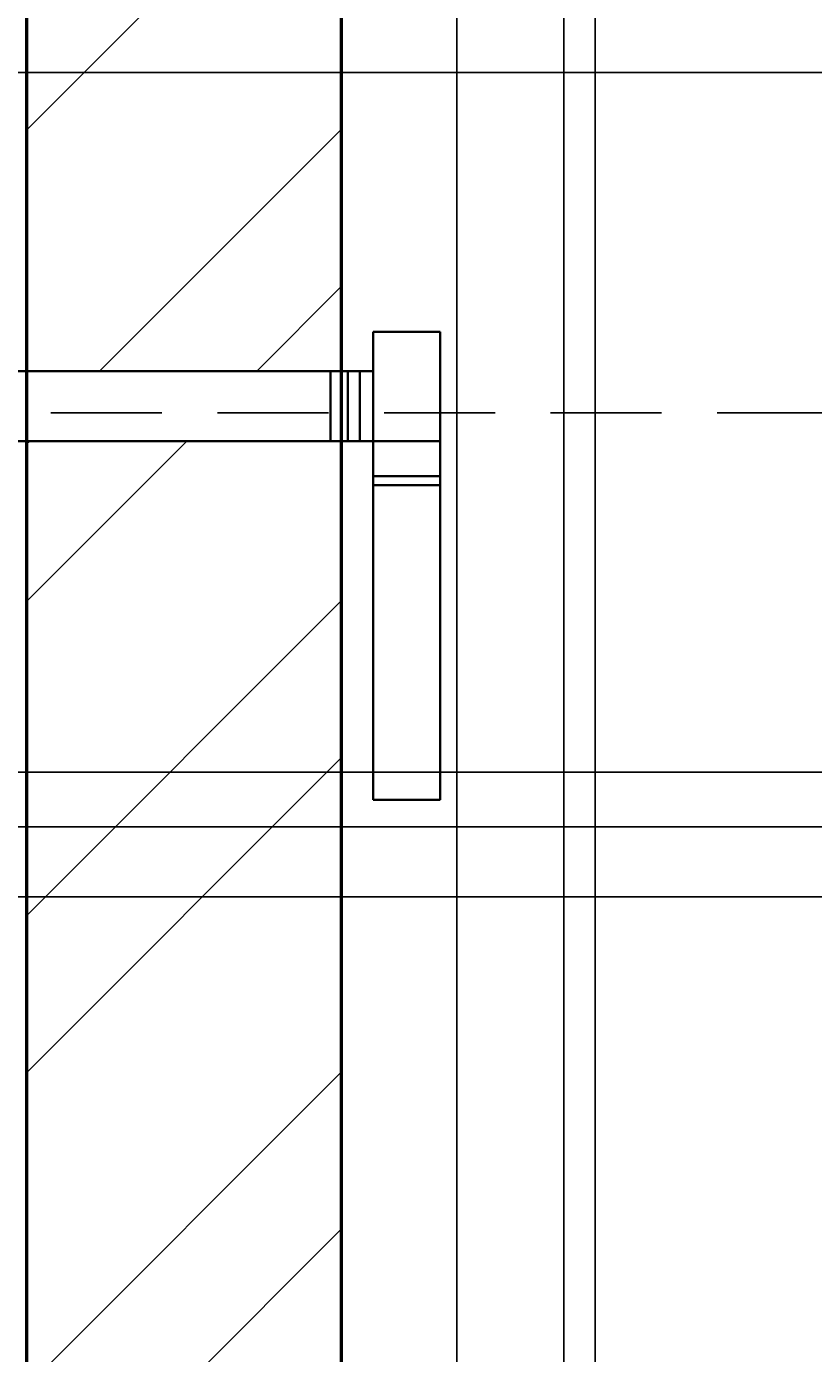
# Model space of a CAD drawing. Units: inches. Extents: x 2812 to 3051, y 1398 to 1659.
# Tile 5 of 65: x 2835 to 2858, y 1435 to 1473. Entities that reach past the tile are written whole.
import ezdxf

# ---------------------------------------------------------------- set-up
doc = ezdxf.new("R2010")
doc.units = ezdxf.units.IN
doc.linetypes.add('HIDDEN2', pattern=[4.7625, 3.175, -1.5875])
for name, color, linetype, lineweight in [('A-ANNO-DIMS', 2, 'Continuous', 18), ('P-SANR-PIPE', 4, 'Continuous', 35), ('S-CONC', 7, 'Continuous', 50), ('S-CONC-HIDN', 8, 'HIDDEN2', 25), ('S-CONC-PATT', 8, 'Continuous', 18)]:
    doc.layers.add(name, color=color, linetype=linetype, lineweight=lineweight)
doc.styles.get("Standard").update_dxf_attribs({"font": 'arial.ttf'})
doc.dimstyles.get("Standard").update_dxf_attribs({"dimtxt": 0.18, "dimasz": 0.18, "dimexe": 0.18, "dimexo": 0.0625, "dimgap": 0.09, "dimtad": 0, "dimtih": 1, "dimtoh": 1, "dimdec": 4, "dimzin": 0, "dimdsep": 46, "dimtxsty": 'Standard', "dimcen": 0.09, "dimadec": 0, "dimazin": 0, "dimtfac": 1, "dimtdec": 4, "dimtofl": 0, "dimtmove": 0, "dimatfit": 3, "dimfxl": 1, "dimtolj": 1, "dimtzin": 0, "dimarcsym": 0})

# ---------------------------------------------------------------- blocks, each defined once
blk = doc.blocks.new('PIPE-TEE-SECTION')
for p, q in [((1.921, 13.381), (0, 13.381)), ((0, 13.381), (0, 12.795)), ((1.921, 12.795), (1.921, 13.381)), ((0, 12.795), (0, 10.254)), ((1.921, 12.235), (1.921, 12.795)), ((2.641, 12.254), (1.921, 12.254)), ((1.921, 10.254), (1.921, 12.235)), ((2.299, 12.254), (2.299, 10.254)), ((2.641, 10.254), (2.641, 12.254)), ((2.641, 12.254), (14.641, 12.254)), ((2.641, 12.254), (3.141, 12.254)), ((3.141, 12.254), (3.141, 10.254)), ((0, 10.254), (1.921, 10.254)), ((0, 10.254), (0, 0)), ((2.299, 10.254), (1.921, 10.254)), ((1.921, 10.254), (1.921, 9.254)), ((14.641, 10.254), (2.299, 10.254)), ((0, 9.254), (1.921, 9.254)), ((0, 9), (0, 9.254)), ((1.921, 9.254), (1.921, 9)), ((1.921, 9), (0, 9)), ((1.921, 9), (1.921, 0)), ((1.921, 0), (0, 0))]:
    blk.add_line(p, q)
blk.add_open_spline([(14.641, 10.254), (14.669, 10.56), (14.725, 11.17), (14.444, 12.118), (14.641, 12.254)], degree=3)
blk = doc.blocks.new('*D28')
at = {"layer": 'A-ANNO-DIMS', "color": 0, "lineweight": -2, "transparency": 16777216}
for p, q in [((2851.646, 1598.667), (2851.646, 1397.505)), ((2844.385, 1559.757), (2844.385, 1397.505)), ((2844.565, 1397.685), (2847.64, 1397.685)), ((2851.466, 1397.685), (2848.391, 1397.685))]:
    blk.add_line(p, q, dxfattribs=at)
at = {"layer": 'A-ANNO-DIMS', "color": 0, "transparency": 16777216}
for points in [[(2844.565, 1397.715), (2844.565, 1397.655), (2844.385, 1397.685)], [(2851.466, 1397.715), (2851.466, 1397.655), (2851.646, 1397.685)]]:
    blk.add_solid(points, dxfattribs=at)
at = {"layer": 'Defpoints', "color": 0, "transparency": 16777216}
for p in [(2851.646, 1598.73), (2844.385, 1559.82), (2851.646, 1397.685)]:
    blk.add_point(p, dxfattribs=at)
at = {"layer": 'A-ANNO-DIMS', "color": 0, "transparency": 16777216, "insert": (2848.016, 1397.685), "char_height": 0.18, "attachment_point": 5}
blk.add_mtext('\\A1;7.261', dxfattribs=at)
blk = doc.blocks.new('*D42')
at = {"layer": 'A-ANNO-DIMS', "color": 0, "lineweight": -2, "transparency": 16777216}
for p, q in [((2828.385, 1489.973), (2828.385, 1397.505)), ((2847.686, 1487.973), (2847.686, 1397.505)), ((2828.565, 1397.685), (2837.72, 1397.685)), ((2847.506, 1397.685), (2838.351, 1397.685))]:
    blk.add_line(p, q, dxfattribs=at)
at = {"layer": 'A-ANNO-DIMS', "color": 0, "transparency": 16777216}
for points in [[(2828.565, 1397.715), (2828.565, 1397.655), (2828.385, 1397.685)], [(2847.506, 1397.715), (2847.506, 1397.655), (2847.686, 1397.685)]]:
    blk.add_solid(points, dxfattribs=at)
at = {"layer": 'Defpoints', "color": 0, "transparency": 16777216}
for p in [(2828.385, 1490.035), (2847.686, 1488.035), (2847.686, 1397.685)]:
    blk.add_point(p, dxfattribs=at)
at = {"layer": 'A-ANNO-DIMS', "color": 0, "transparency": 16777216, "insert": (2838.036, 1397.685), "char_height": 0.18, "attachment_point": 5}
blk.add_mtext('\\A1;19.3', dxfattribs=at)
blk = doc.blocks.new('*D43')
at = {"layer": 'A-ANNO-DIMS', "color": 0, "lineweight": -2, "transparency": 16777216}
for p, q in [((2847.686, 1487.973), (2847.686, 1397.505)), ((2850.748, 1487.973), (2850.748, 1397.505)), ((2847.866, 1397.685), (2848.825, 1397.685)), ((2850.568, 1397.685), (2849.61, 1397.685))]:
    blk.add_line(p, q, dxfattribs=at)
at = {"layer": 'A-ANNO-DIMS', "color": 0, "transparency": 16777216}
for points in [[(2847.866, 1397.715), (2847.866, 1397.655), (2847.686, 1397.685)], [(2850.568, 1397.715), (2850.568, 1397.655), (2850.748, 1397.685)]]:
    blk.add_solid(points, dxfattribs=at)
at = {"layer": 'Defpoints', "color": 0, "transparency": 16777216}
for p in [(2847.686, 1488.035), (2850.748, 1488.035), (2850.748, 1397.685)]:
    blk.add_point(p, dxfattribs=at)
at = {"layer": 'A-ANNO-DIMS', "color": 0, "transparency": 16777216, "insert": (2849.217, 1397.685), "char_height": 0.18, "attachment_point": 5}
blk.add_mtext('\\A1;3.062', dxfattribs=at)
blk = doc.blocks.new('*D44')
at = {"layer": 'A-ANNO-DIMS', "color": 0, "lineweight": -2, "transparency": 16777216}
for p, q in [((2850.748, 1487.973), (2850.748, 1397.505)), ((2896.385, 1487.973), (2896.385, 1397.505)), ((2850.928, 1397.685), (2873.17, 1397.685)), ((2896.205, 1397.685), (2873.964, 1397.685))]:
    blk.add_line(p, q, dxfattribs=at)
at = {"layer": 'A-ANNO-DIMS', "color": 0, "transparency": 16777216}
for points in [[(2850.928, 1397.715), (2850.928, 1397.655), (2850.748, 1397.685)], [(2896.205, 1397.715), (2896.205, 1397.655), (2896.385, 1397.685)]]:
    blk.add_solid(points, dxfattribs=at)
at = {"layer": 'Defpoints', "color": 0, "transparency": 16777216}
for p in [(2850.748, 1488.035), (2896.385, 1488.035), (2896.385, 1397.685)]:
    blk.add_point(p, dxfattribs=at)
at = {"layer": 'A-ANNO-DIMS', "color": 0, "transparency": 16777216, "insert": (2873.567, 1397.685), "char_height": 0.18, "attachment_point": 5}
blk.add_mtext('\\A1;45.64', dxfattribs=at)
blk = doc.blocks.new('*D56')
at = {"layer": 'A-ANNO-DIMS', "color": 0, "lineweight": -2, "transparency": 16777216}
for p, q in [((2880.322, 1452.035), (2811.806, 1452.035)), ((2811.986, 1451.855), (2811.986, 1434.217)), ((2811.986, 1416.215), (2811.986, 1433.853)), ((2952.322, 1416.035), (2811.806, 1416.035))]:
    blk.add_line(p, q, dxfattribs=at)
at = {"layer": 'A-ANNO-DIMS', "color": 0, "transparency": 16777216}
for points in [[(2811.956, 1451.855), (2812.016, 1451.855), (2811.986, 1452.035)], [(2811.956, 1416.215), (2812.016, 1416.215), (2811.986, 1416.035)]]:
    blk.add_solid(points, dxfattribs=at)
at = {"layer": 'Defpoints', "color": 0, "transparency": 16777216}
for p in [(2811.986, 1452.035), (2880.385, 1452.035), (2952.385, 1416.035)]:
    blk.add_point(p, dxfattribs=at)
at = {"layer": 'A-ANNO-DIMS', "color": 0, "transparency": 16777216, "insert": (2811.986, 1434.035), "char_height": 0.18, "attachment_point": 5}
blk.add_mtext('\\A1;36', dxfattribs=at)
blk = doc.blocks.new('*D57')
at = {"layer": 'A-ANNO-DIMS', "color": 0, "lineweight": -2, "transparency": 16777216}
for p, q in [((2880.322, 1472.035), (2811.806, 1472.035)), ((2811.986, 1471.855), (2811.986, 1462.217)), ((2811.986, 1452.215), (2811.986, 1461.853)), ((2880.322, 1452.035), (2811.806, 1452.035))]:
    blk.add_line(p, q, dxfattribs=at)
at = {"layer": 'A-ANNO-DIMS', "color": 0, "transparency": 16777216}
for points in [[(2811.956, 1471.855), (2812.016, 1471.855), (2811.986, 1472.035)], [(2811.956, 1452.215), (2812.016, 1452.215), (2811.986, 1452.035)]]:
    blk.add_solid(points, dxfattribs=at)
at = {"layer": 'Defpoints', "color": 0, "transparency": 16777216}
for p in [(2811.986, 1472.035), (2880.385, 1472.035), (2880.385, 1452.035)]:
    blk.add_point(p, dxfattribs=at)
at = {"layer": 'A-ANNO-DIMS', "color": 0, "transparency": 16777216, "insert": (2811.986, 1462.035), "char_height": 0.18, "attachment_point": 5}
blk.add_mtext('\\A1;20', dxfattribs=at)
blk = doc.blocks.new('*D75')
at = {"layer": 'A-ANNO-DIMS', "color": 0, "lineweight": -2, "transparency": 16777216}
for p, q in [((2963.812, 1448.474), (2811.806, 1448.474)), ((2811.986, 1448.294), (2811.986, 1432.437)), ((2811.986, 1416.215), (2811.986, 1432.073)), ((2961.322, 1416.035), (2811.806, 1416.035))]:
    blk.add_line(p, q, dxfattribs=at)
at = {"layer": 'A-ANNO-DIMS', "color": 0, "transparency": 16777216}
for points in [[(2811.956, 1448.294), (2812.016, 1448.294), (2811.986, 1448.474)], [(2811.956, 1416.215), (2812.016, 1416.215), (2811.986, 1416.035)]]:
    blk.add_solid(points, dxfattribs=at)
at = {"layer": 'Defpoints', "color": 0, "transparency": 16777216}
for p in [(2811.986, 1448.474), (2963.874, 1448.474), (2961.385, 1416.035)]:
    blk.add_point(p, dxfattribs=at)
at = {"layer": 'A-ANNO-DIMS', "color": 0, "transparency": 16777216, "insert": (2811.986, 1432.255), "char_height": 0.18, "attachment_point": 5}
blk.add_mtext('\\A1;32.44', dxfattribs=at)
blk = doc.blocks.new('*D76')
at = {"layer": 'A-ANNO-DIMS', "color": 0, "lineweight": -2, "transparency": 16777216}
for p, q in [((2963.812, 1450.474), (2811.806, 1450.474)), ((2811.986, 1450.294), (2811.986, 1449.654)), ((2811.986, 1448.654), (2811.986, 1449.293)), ((2963.812, 1448.474), (2811.806, 1448.474))]:
    blk.add_line(p, q, dxfattribs=at)
at = {"layer": 'A-ANNO-DIMS', "color": 0, "transparency": 16777216}
for points in [[(2811.956, 1450.294), (2812.016, 1450.294), (2811.986, 1450.474)], [(2811.956, 1448.654), (2812.016, 1448.654), (2811.986, 1448.474)]]:
    blk.add_solid(points, dxfattribs=at)
at = {"layer": 'Defpoints', "color": 0, "transparency": 16777216}
for p in [(2811.986, 1450.474), (2963.874, 1450.474), (2963.874, 1448.474)]:
    blk.add_point(p, dxfattribs=at)
at = {"layer": 'A-ANNO-DIMS', "color": 0, "transparency": 16777216, "insert": (2811.986, 1449.474), "char_height": 0.18, "attachment_point": 5}
blk.add_mtext('\\A1;2', dxfattribs=at)
blk = doc.blocks.new('*D77')
at = {"layer": 'A-ANNO-DIMS', "color": 0, "lineweight": -2, "transparency": 16777216}
for p, q in [((2961.322, 1472.035), (2811.806, 1472.035)), ((2811.986, 1471.855), (2811.986, 1461.436)), ((2811.986, 1450.654), (2811.986, 1461.073)), ((2963.812, 1450.474), (2811.806, 1450.474))]:
    blk.add_line(p, q, dxfattribs=at)
at = {"layer": 'A-ANNO-DIMS', "color": 0, "transparency": 16777216}
for points in [[(2811.956, 1471.855), (2812.016, 1471.855), (2811.986, 1472.035)], [(2811.956, 1450.654), (2812.016, 1450.654), (2811.986, 1450.474)]]:
    blk.add_solid(points, dxfattribs=at)
at = {"layer": 'Defpoints', "color": 0, "transparency": 16777216}
for p in [(2811.986, 1472.035), (2961.385, 1472.035), (2963.874, 1450.474)]:
    blk.add_point(p, dxfattribs=at)
at = {"layer": 'A-ANNO-DIMS', "color": 0, "transparency": 16777216, "insert": (2811.986, 1461.255), "char_height": 0.18, "attachment_point": 5}
blk.add_mtext('\\A1;21.56', dxfattribs=at)

msp = doc.modelspace()

# ---------------------------------------------------------------- hatches: boundary and pattern name
at = {"layer": 'S-CONC-PATT'}
h = msp.add_hatch(dxfattribs=at)
h.set_pattern_fill('ANSI32', color=256)
h.paths.add_polyline_path([(3027.3849, 1646.82), (2835.3849, 1646.82), (2835.3849, 1603.2296), (2844.3849, 1603.2296), (2844.3849, 1637.82), (3018.3849, 1637.82), (3018.3849, 1602.5441), (3027.3849, 1602.5441)])
h.paths.add_polyline_path([(2844.3849, 1594.2296), (2835.3849, 1594.2296), (2835.3849, 1550.82), (3027.3849, 1550.82), (3027.3849, 1593.5441), (3018.3849, 1593.5441), (3018.3849, 1559.82), (2844.3849, 1559.82)])
h.paths.add_polyline_path([(2844.3849, 1482.0354), (2835.3849, 1482.0354), (2835.3849, 1463.4959), (2844.3849, 1463.4959)])
h.paths.add_polyline_path([(2844.3849, 1461.4959), (2835.3849, 1461.4959), (2835.3849, 1416.0354), (2844.3849, 1416.0354)])
h.paths.add_polyline_path([(3027.3849, 1482.0354), (3018.3849, 1482.0354), (3018.3849, 1463.2854), (3027.3849, 1463.2854)])
h.paths.add_polyline_path([(3027.3849, 1461.2854), (3018.3849, 1461.2854), (3018.3849, 1416.0354), (3027.3849, 1416.0354)])
h.paths.add_polyline_path([(2961.3849, 1448.4738), (2952.3849, 1448.4738), (2952.3849, 1416.0354), (2961.3849, 1416.0354)])
h.paths.add_polyline_path([(2961.3849, 1462.3026), (2952.3849, 1462.3026), (2952.3849, 1450.4738), (2961.3849, 1450.4738)])
h.paths.add_polyline_path([(2961.3849, 1472.0354), (2952.3849, 1472.0354), (2952.3849, 1462.3026), (2961.3849, 1462.3026)])

# ---------------------------------------------------------------- linework, layer by layer
at = {"layer": 'S-CONC'}
for p, q in [((2835.3849, 1482.0354), (2835.3849, 1416.0354)), ((2835.3849, 1482.0354), (2835.3849, 1416.0354)), ((2844.3849, 1482.0354), (2844.3849, 1416.0354))]:
    msp.add_line(p, q, dxfattribs=at)
at = {"layer": 'S-CONC-HIDN'}
msp.add_line((3029.7562, 1462.3026), (2835.3849, 1462.3026), dxfattribs=at)

# ---------------------------------------------------------------- block references
at = {"layer": 'P-SANR-PIPE', "extrusion": (0, 0, -1), "zscale": -1}
msp.add_blockref('PIPE-TEE-SECTION', (-2847.2154, 1451.2415), dxfattribs=at)

# ---------------------------------------------------------------- dimensions: what is measured, and where the dimension line sits
at = {"layer": 'A-ANNO-DIMS'}
for base, p1, p2, override, picture, middle in [((2851.6462, 1397.6854), (2844.3849, 1559.82), (2851.6462, 1598.7296), {"dimdec": 3, "dimlfac": 1, "dimrnd": 0, "dimzin": 0, "dimdsep": 46, "dimlunit": 2}, '*D28', (2848.0156, 1397.6854)), ((2847.6863, 1397.6854), (2828.3849, 1490.0354), (2847.6863, 1488.0354), {"dimdec": 1, "dimlfac": 1, "dimrnd": 0, "dimzin": 0, "dimdsep": 46, "dimlunit": 2}, '*D42', (2838.0356, 1397.6854)), ((2850.7485, 1397.6854), (2847.6863, 1488.0354), (2850.7485, 1488.0354), {"dimdec": 3, "dimlfac": 1, "dimrnd": 0, "dimzin": 0, "dimdsep": 46, "dimlunit": 2}, '*D43', (2849.2174, 1397.6854)), ((2896.3849, 1397.6854), (2850.7485, 1488.0354), (2896.3849, 1488.0354), {"dimdec": 2, "dimlfac": 1, "dimrnd": 0, "dimzin": 0, "dimdsep": 46, "dimlunit": 2}, '*D44', (2873.5667, 1397.6854))]:
    dim = msp.add_linear_dim(base=base, p1=p1, p2=p2, dimstyle='Standard', override=override, dxfattribs=at)
    dim.commit()
    dim.dimension.update_dxf_attribs({"geometry": picture, "text_midpoint": middle})
for base, p1, p2, override, picture, middle in [((2811.9855, 1472.0354), (2963.8741, 1450.4738), (2961.3849, 1472.0354), {"dimdec": 2, "dimlfac": 1, "dimrnd": 0, "dimzin": 0, "dimdsep": 46, "dimlunit": 2}, '*D77', (2811.9855, 1461.2546)), ((2811.9855, 1472.0354), (2880.3849, 1452.0354), (2880.3849, 1472.0354), {"dimdec": 0, "dimlfac": 1, "dimrnd": 0, "dimzin": 0, "dimdsep": 46, "dimlunit": 2}, '*D57', (2811.9855, 1462.0354)), ((2811.9855, 1452.0354), (2952.3849, 1416.0354), (2880.3849, 1452.0354), {"dimdec": 0, "dimlfac": 1, "dimrnd": 0, "dimzin": 0, "dimdsep": 46, "dimlunit": 2}, '*D56', (2811.9855, 1434.0354)), ((2811.9855, 1450.4738), (2963.8741, 1448.4738), (2963.8741, 1450.4738), {"dimdec": 0, "dimlfac": 1, "dimrnd": 0, "dimzin": 0, "dimdsep": 46, "dimlunit": 2}, '*D76', (2811.9855, 1449.4738)), ((2811.9855, 1448.4738), (2961.3849, 1416.0354), (2963.8741, 1448.4738), {"dimdec": 2, "dimlfac": 1, "dimrnd": 0, "dimzin": 0, "dimdsep": 46, "dimlunit": 2}, '*D75', (2811.9855, 1432.2546))]:
    dim = msp.add_linear_dim(base=base, p1=p1, p2=p2, angle=90, dimstyle='Standard', override=override, dxfattribs=at)
    dim.commit()
    dim.dimension.update_dxf_attribs({"geometry": picture, "text_midpoint": middle})

doc.saveas('drawing.dxf')
